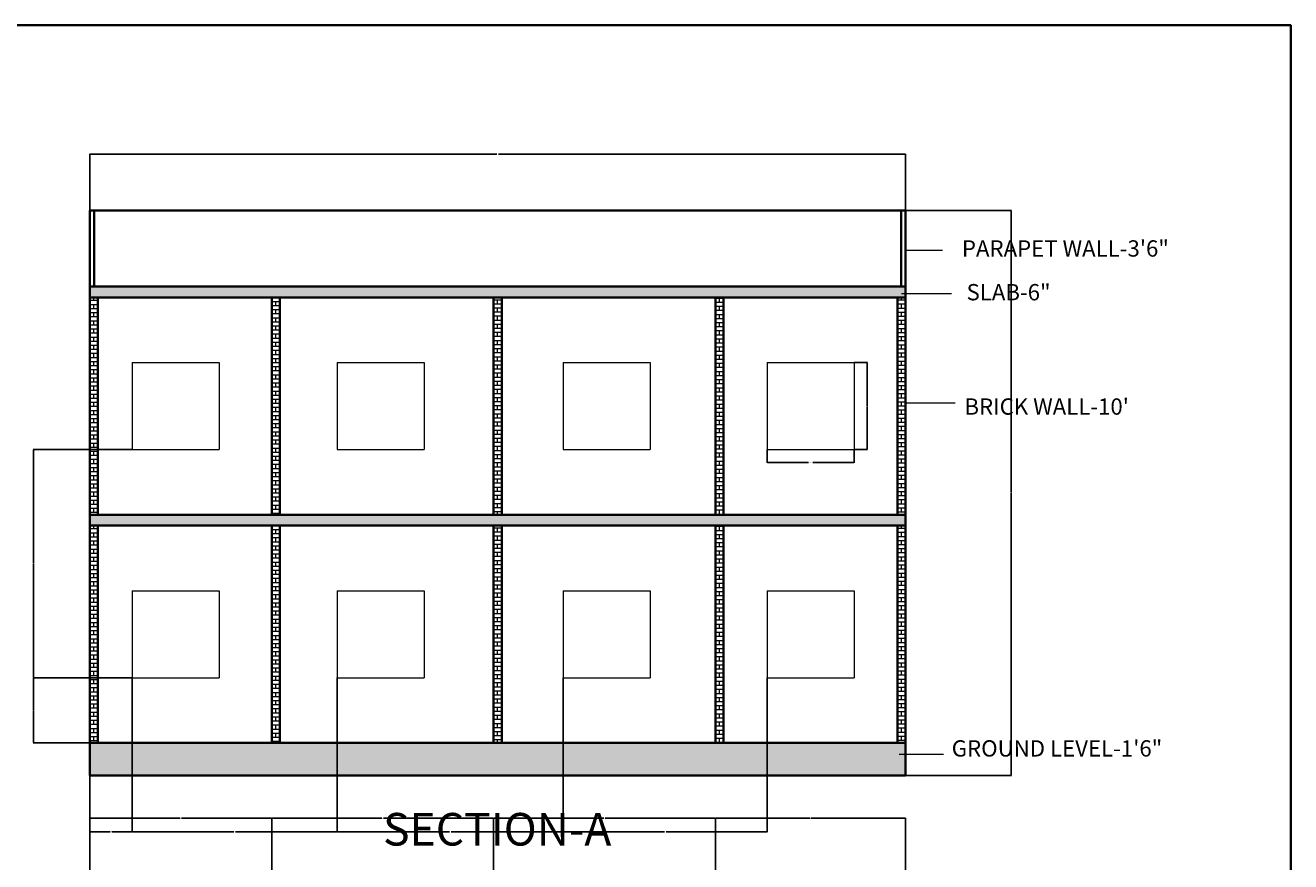
# Model space of a CAD drawing. Units: inches. Extents: x 2043 to 3387, y 1535 to 2797.
# Tile 7 of 7: x 2688 to 3387, y 2335 to 2797. Entities that reach past the tile are written whole.
import ezdxf

# ---------------------------------------------------------------- set-up
doc = ezdxf.new("R2010")
doc.units = ezdxf.units.IN
for name, color, linetype, lineweight in [('A-ANNO-DIMS', 2, 'Continuous', 18), ('A-ANNO-TEXT', 7, 'Continuous', 18), ('A-ANNO-TITL', 7, 'Continuous', 30), ('A-ANNO-TTLB', 7, 'Continuous', 35), ('A-GLAZ', 4, 'Continuous', 18), ('A-SECT', 7, 'Continuous', 35), ('A-WALL-PATT', 8, 'Continuous', 13), ('S-CONC-PATT', 8, 'Continuous', 13)]:
    doc.layers.add(name, color=color, linetype=linetype, lineweight=lineweight)
doc.styles.get("Standard").update_dxf_attribs({"font": 'arial.ttf'})
doc.dimstyles.get("Standard").update_dxf_attribs({"dimtxt": 0.18, "dimasz": 0.18, "dimexe": 0.18, "dimexo": 0.0625, "dimgap": 0.09, "dimtad": 0, "dimtih": 1, "dimtoh": 1, "dimdec": 4, "dimzin": 0, "dimdsep": 46, "dimtxsty": 'Standard', "dimcen": 0.09, "dimadec": 0, "dimazin": 0, "dimtfac": 1, "dimtdec": 4, "dimtofl": 0, "dimtmove": 0, "dimatfit": 3, "dimfxl": 1, "dimtolj": 1, "dimtzin": 0, "dimarcsym": 0})

# ---------------------------------------------------------------- blocks, each defined once
blk = doc.blocks.new('WIN-48-SECTION')
for p, q in [((0, 48), (48, 48)), ((0, 48), (0, 0)), ((48, 48), (48, 0)), ((0, 0), (48, 0))]:
    blk.add_line(p, q)
blk = doc.blocks.new('*D47')
at = {"layer": 'A-ANNO-DIMS', "color": 0, "lineweight": -2, "transparency": 16777216}
for p, q in [((3097.86, 2562.49), (3097.86, 2555.17)), ((3145.86, 2562.49), (3145.86, 2555.17)), ((3098.04, 2555.35), (3120.72, 2555.35)), ((3145.68, 2555.35), (3123, 2555.35))]:
    blk.add_line(p, q, dxfattribs=at)
at = {"layer": 'A-ANNO-DIMS', "color": 0, "transparency": 16777216}
for points in [[(3098.04, 2555.38), (3098.04, 2555.32), (3097.86, 2555.35)], [(3145.68, 2555.38), (3145.68, 2555.32), (3145.86, 2555.35)]]:
    blk.add_solid(points, dxfattribs=at)
at = {"layer": 'Defpoints', "color": 0, "transparency": 16777216}
for p in [(3097.86, 2562.55), (3145.86, 2562.55), (3145.86, 2555.35)]:
    blk.add_point(p, dxfattribs=at)
at = {"layer": 'A-ANNO-DIMS', "color": 0, "transparency": 16777216, "insert": (3121.86, 2555.35), "char_height": 0.18, "attachment_point": 5}
blk.add_mtext('\\A1;OPENING 48 TYP.', dxfattribs=at)
blk = doc.blocks.new('*D48')
at = {"layer": 'A-ANNO-DIMS', "color": 0, "lineweight": -2, "transparency": 16777216}
for p, q in [((3145.92, 2610.55), (3153.24, 2610.55)), ((3153.06, 2610.37), (3153.06, 2586.73)), ((3153.06, 2562.73), (3153.06, 2586.37)), ((3145.92, 2562.55), (3153.24, 2562.55))]:
    blk.add_line(p, q, dxfattribs=at)
at = {"layer": 'A-ANNO-DIMS', "color": 0, "transparency": 16777216}
for points in [[(3153.03, 2610.37), (3153.09, 2610.37), (3153.06, 2610.55)], [(3153.03, 2562.73), (3153.09, 2562.73), (3153.06, 2562.55)]]:
    blk.add_solid(points, dxfattribs=at)
at = {"layer": 'Defpoints', "color": 0, "transparency": 16777216}
for p in [(3145.86, 2610.55), (3153.06, 2610.55), (3145.86, 2562.55)]:
    blk.add_point(p, dxfattribs=at)
at = {"layer": 'A-ANNO-DIMS', "color": 0, "transparency": 16777216, "insert": (3153.06, 2586.55), "char_height": 0.18, "attachment_point": 5}
blk.add_mtext('\\A1;48 TYP.', dxfattribs=at)
blk = doc.blocks.new('*D107')
at = {"layer": 'A-ANNO-DIMS', "color": 0, "lineweight": -2, "transparency": 16777216}
for p, q in [((2723.71, 2326.44), (2723.71, 2359.26)), ((2723.89, 2359.08), (2773.57, 2359.08)), ((2824.03, 2359.08), (2774.34, 2359.08)), ((2824.21, 2317.44), (2824.21, 2359.26))]:
    blk.add_line(p, q, dxfattribs=at)
at = {"layer": 'A-ANNO-DIMS', "color": 0, "transparency": 16777216}
for points in [[(2723.89, 2359.11), (2723.89, 2359.05), (2723.71, 2359.08)], [(2824.03, 2359.11), (2824.03, 2359.05), (2824.21, 2359.08)]]:
    blk.add_solid(points, dxfattribs=at)
at = {"layer": 'Defpoints', "color": 0, "transparency": 16777216}
for p in [(2824.21, 2359.08), (2723.71, 2326.38), (2824.21, 2317.38)]:
    blk.add_point(p, dxfattribs=at)
at = {"layer": 'A-ANNO-DIMS', "color": 0, "transparency": 16777216, "insert": (2773.96, 2359.08), "char_height": 0.18, "attachment_point": 5}
blk.add_mtext('\\A1;100.5', dxfattribs=at)
blk = doc.blocks.new('*D108')
at = {"layer": 'A-ANNO-DIMS', "color": 0, "lineweight": -2, "transparency": 16777216}
for p, q in [((2824.21, 2317.44), (2824.21, 2359.26)), ((2824.39, 2359.08), (2885.07, 2359.08)), ((2946.53, 2359.08), (2885.84, 2359.08)), ((2946.71, 2317.44), (2946.71, 2359.26))]:
    blk.add_line(p, q, dxfattribs=at)
at = {"layer": 'A-ANNO-DIMS', "color": 0, "transparency": 16777216}
for points in [[(2824.39, 2359.11), (2824.39, 2359.05), (2824.21, 2359.08)], [(2946.53, 2359.11), (2946.53, 2359.05), (2946.71, 2359.08)]]:
    blk.add_solid(points, dxfattribs=at)
at = {"layer": 'Defpoints', "color": 0, "transparency": 16777216}
for p in [(2946.71, 2359.08), (2824.21, 2317.38), (2946.71, 2317.38)]:
    blk.add_point(p, dxfattribs=at)
at = {"layer": 'A-ANNO-DIMS', "color": 0, "transparency": 16777216, "insert": (2885.46, 2359.08), "char_height": 0.18, "attachment_point": 5}
blk.add_mtext('\\A1;122.5', dxfattribs=at)
blk = doc.blocks.new('*D109')
at = {"layer": 'A-ANNO-DIMS', "color": 0, "lineweight": -2, "transparency": 16777216}
for p, q in [((2946.71, 2317.44), (2946.71, 2359.26)), ((2946.89, 2359.08), (3007.57, 2359.08)), ((3069.03, 2359.08), (3008.34, 2359.08)), ((3069.21, 2317.44), (3069.21, 2359.26))]:
    blk.add_line(p, q, dxfattribs=at)
at = {"layer": 'A-ANNO-DIMS', "color": 0, "transparency": 16777216}
for points in [[(2946.89, 2359.11), (2946.89, 2359.05), (2946.71, 2359.08)], [(3069.03, 2359.11), (3069.03, 2359.05), (3069.21, 2359.08)]]:
    blk.add_solid(points, dxfattribs=at)
at = {"layer": 'Defpoints', "color": 0, "transparency": 16777216}
for p in [(3069.21, 2359.08), (2946.71, 2317.38), (3069.21, 2317.38)]:
    blk.add_point(p, dxfattribs=at)
at = {"layer": 'A-ANNO-DIMS', "color": 0, "transparency": 16777216, "insert": (3007.96, 2359.08), "char_height": 0.18, "attachment_point": 5}
blk.add_mtext('\\A1;122.5', dxfattribs=at)
blk = doc.blocks.new('*D110')
at = {"layer": 'A-ANNO-DIMS', "color": 0, "lineweight": -2, "transparency": 16777216}
for p, q in [((3069.21, 2317.44), (3069.21, 2359.26)), ((3069.39, 2359.08), (3121.43, 2359.08)), ((3174.03, 2359.08), (3121.99, 2359.08)), ((3174.21, 2326.44), (3174.21, 2359.26))]:
    blk.add_line(p, q, dxfattribs=at)
at = {"layer": 'A-ANNO-DIMS', "color": 0, "transparency": 16777216}
for points in [[(3069.39, 2359.11), (3069.39, 2359.05), (3069.21, 2359.08)], [(3174.03, 2359.11), (3174.03, 2359.05), (3174.21, 2359.08)]]:
    blk.add_solid(points, dxfattribs=at)
at = {"layer": 'Defpoints', "color": 0, "transparency": 16777216}
for p in [(3174.21, 2359.08), (3174.21, 2326.38), (3069.21, 2317.38)]:
    blk.add_point(p, dxfattribs=at)
at = {"layer": 'A-ANNO-DIMS', "color": 0, "transparency": 16777216, "insert": (3121.71, 2359.08), "char_height": 0.18, "attachment_point": 5}
blk.add_mtext('\\A1;105', dxfattribs=at)
blk = doc.blocks.new('*D120')
at = {"layer": 'A-ANNO-DIMS', "color": 0, "lineweight": -2, "transparency": 16777216}
for p, q in [((2723.71, 2694.61), (2723.71, 2725.78)), ((3174.21, 2694.61), (3174.21, 2725.78)), ((2723.89, 2725.6), (2948.56, 2725.6)), ((3174.03, 2725.6), (2949.36, 2725.6))]:
    blk.add_line(p, q, dxfattribs=at)
at = {"layer": 'A-ANNO-DIMS', "color": 0, "transparency": 16777216}
for points in [[(2723.89, 2725.63), (2723.89, 2725.57), (2723.71, 2725.6)], [(3174.03, 2725.63), (3174.03, 2725.57), (3174.21, 2725.6)]]:
    blk.add_solid(points, dxfattribs=at)
at = {"layer": 'Defpoints', "color": 0, "transparency": 16777216}
for p in [(3174.21, 2725.6), (2723.71, 2694.55), (3174.21, 2694.55)]:
    blk.add_point(p, dxfattribs=at)
at = {"layer": 'A-ANNO-DIMS', "color": 0, "transparency": 16777216, "insert": (2948.96, 2725.6), "char_height": 0.18, "attachment_point": 5}
blk.add_mtext('\\A1;450.5', dxfattribs=at)
blk = doc.blocks.new('*D121')
at = {"layer": 'A-ANNO-DIMS', "color": 0, "lineweight": -2, "transparency": 16777216}
for p, q in [((3174.27, 2694.55), (3232.83, 2694.55)), ((3232.65, 2694.37), (3232.65, 2538.73)), ((3232.65, 2382.73), (3232.65, 2538.37)), ((3174.27, 2382.55), (3232.83, 2382.55))]:
    blk.add_line(p, q, dxfattribs=at)
at = {"layer": 'A-ANNO-DIMS', "color": 0, "transparency": 16777216}
for points in [[(3232.62, 2694.37), (3232.68, 2694.37), (3232.65, 2694.55)], [(3232.62, 2382.73), (3232.68, 2382.73), (3232.65, 2382.55)]]:
    blk.add_solid(points, dxfattribs=at)
at = {"layer": 'Defpoints', "color": 0, "transparency": 16777216}
for p in [(3174.21, 2694.55), (3232.65, 2694.55), (3174.21, 2382.55)]:
    blk.add_point(p, dxfattribs=at)
at = {"layer": 'A-ANNO-DIMS', "color": 0, "transparency": 16777216, "insert": (3232.65, 2538.55), "char_height": 0.18, "attachment_point": 5}
blk.add_mtext('\\A1;312', dxfattribs=at)
blk = doc.blocks.new('*D127')
at = {"layer": 'A-ANNO-DIMS', "color": 0, "lineweight": -2, "transparency": 16777216}
for p, q in [((2747.01, 2562.55), (2692.48, 2562.55)), ((2692.66, 2562.37), (2692.66, 2499.73)), ((2692.66, 2436.73), (2692.66, 2499.37)), ((2747.01, 2436.55), (2692.48, 2436.55))]:
    blk.add_line(p, q, dxfattribs=at)
at = {"layer": 'A-ANNO-DIMS', "color": 0, "transparency": 16777216}
for points in [[(2692.63, 2562.37), (2692.69, 2562.37), (2692.66, 2562.55)], [(2692.63, 2436.73), (2692.69, 2436.73), (2692.66, 2436.55)]]:
    blk.add_solid(points, dxfattribs=at)
at = {"layer": 'Defpoints', "color": 0, "transparency": 16777216}
for p in [(2692.66, 2562.55), (2747.07, 2562.55), (2747.07, 2436.55)]:
    blk.add_point(p, dxfattribs=at)
at = {"layer": 'A-ANNO-DIMS', "color": 0, "transparency": 16777216, "insert": (2692.66, 2499.55), "char_height": 0.18, "attachment_point": 5}
blk.add_mtext('\\A1;126', dxfattribs=at)
blk = doc.blocks.new('*D128')
at = {"layer": 'A-ANNO-DIMS', "color": 0, "lineweight": -2, "transparency": 16777216}
for p, q in [((2747.07, 2436.49), (2747.07, 2351.32)), ((2723.71, 2400.49), (2723.71, 2351.32)), ((2723.89, 2351.5), (2734.99, 2351.5)), ((2746.89, 2351.5), (2735.78, 2351.5))]:
    blk.add_line(p, q, dxfattribs=at)
at = {"layer": 'A-ANNO-DIMS', "color": 0, "transparency": 16777216}
for points in [[(2723.89, 2351.53), (2723.89, 2351.47), (2723.71, 2351.5)], [(2746.89, 2351.53), (2746.89, 2351.47), (2747.07, 2351.5)]]:
    blk.add_solid(points, dxfattribs=at)
at = {"layer": 'Defpoints', "color": 0, "transparency": 16777216}
for p in [(2747.07, 2436.55), (2723.71, 2400.55), (2747.07, 2351.5)]:
    blk.add_point(p, dxfattribs=at)
at = {"layer": 'A-ANNO-DIMS', "color": 0, "transparency": 16777216, "insert": (2735.39, 2351.5), "char_height": 0.18, "attachment_point": 5}
blk.add_mtext('\\A1;23.36', dxfattribs=at)
blk = doc.blocks.new('*D129')
at = {"layer": 'A-ANNO-DIMS', "color": 0, "lineweight": -2, "transparency": 16777216}
for p, q in [((2747.07, 2436.49), (2747.07, 2351.32)), ((2860.38, 2436.49), (2860.38, 2351.32)), ((2747.25, 2351.5), (2803.29, 2351.5)), ((2860.2, 2351.5), (2804.16, 2351.5))]:
    blk.add_line(p, q, dxfattribs=at)
at = {"layer": 'A-ANNO-DIMS', "color": 0, "transparency": 16777216}
for points in [[(2747.25, 2351.53), (2747.25, 2351.47), (2747.07, 2351.5)], [(2860.2, 2351.53), (2860.2, 2351.47), (2860.38, 2351.5)]]:
    blk.add_solid(points, dxfattribs=at)
at = {"layer": 'Defpoints', "color": 0, "transparency": 16777216}
for p in [(2747.07, 2436.55), (2860.38, 2436.55), (2860.38, 2351.5)]:
    blk.add_point(p, dxfattribs=at)
at = {"layer": 'A-ANNO-DIMS', "color": 0, "transparency": 16777216, "insert": (2803.73, 2351.5), "char_height": 0.18, "attachment_point": 5}
blk.add_mtext('\\A1;113.31', dxfattribs=at)
blk = doc.blocks.new('*D130')
at = {"layer": 'A-ANNO-DIMS', "color": 0, "lineweight": -2, "transparency": 16777216}
for p, q in [((2860.38, 2436.49), (2860.38, 2351.32)), ((2985.21, 2436.49), (2985.21, 2351.32)), ((2860.56, 2351.5), (2922.34, 2351.5)), ((2985.03, 2351.5), (2923.25, 2351.5))]:
    blk.add_line(p, q, dxfattribs=at)
at = {"layer": 'A-ANNO-DIMS', "color": 0, "transparency": 16777216}
for points in [[(2860.56, 2351.53), (2860.56, 2351.47), (2860.38, 2351.5)], [(2985.03, 2351.53), (2985.03, 2351.47), (2985.21, 2351.5)]]:
    blk.add_solid(points, dxfattribs=at)
at = {"layer": 'Defpoints', "color": 0, "transparency": 16777216}
for p in [(2860.38, 2436.55), (2985.21, 2436.55), (2985.21, 2351.5)]:
    blk.add_point(p, dxfattribs=at)
at = {"layer": 'A-ANNO-DIMS', "color": 0, "transparency": 16777216, "insert": (2922.8, 2351.5), "char_height": 0.18, "attachment_point": 5}
blk.add_mtext('\\A1;124.83', dxfattribs=at)
blk = doc.blocks.new('*D131')
at = {"layer": 'A-ANNO-DIMS', "color": 0, "lineweight": -2, "transparency": 16777216}
for p, q in [((2985.21, 2436.49), (2985.21, 2351.32)), ((3097.86, 2436.49), (3097.86, 2351.32)), ((2985.39, 2351.5), (3041.08, 2351.5)), ((3097.68, 2351.5), (3041.99, 2351.5))]:
    blk.add_line(p, q, dxfattribs=at)
at = {"layer": 'A-ANNO-DIMS', "color": 0, "transparency": 16777216}
for points in [[(2985.39, 2351.53), (2985.39, 2351.47), (2985.21, 2351.5)], [(3097.68, 2351.53), (3097.68, 2351.47), (3097.86, 2351.5)]]:
    blk.add_solid(points, dxfattribs=at)
at = {"layer": 'Defpoints', "color": 0, "transparency": 16777216}
for p in [(2985.21, 2436.55), (3097.86, 2436.55), (3097.86, 2351.5)]:
    blk.add_point(p, dxfattribs=at)
at = {"layer": 'A-ANNO-DIMS', "color": 0, "transparency": 16777216, "insert": (3041.54, 2351.5), "char_height": 0.18, "attachment_point": 5}
blk.add_mtext('\\A1;112.65', dxfattribs=at)
blk = doc.blocks.new('*D132')
at = {"layer": 'A-ANNO-DIMS', "color": 0, "lineweight": -2, "transparency": 16777216}
for p, q in [((2747.01, 2436.55), (2692.48, 2436.55)), ((2692.66, 2436.37), (2692.66, 2418.73)), ((2692.66, 2400.73), (2692.66, 2418.37)), ((2723.65, 2400.55), (2692.48, 2400.55))]:
    blk.add_line(p, q, dxfattribs=at)
at = {"layer": 'A-ANNO-DIMS', "color": 0, "transparency": 16777216}
for points in [[(2692.63, 2436.37), (2692.69, 2436.37), (2692.66, 2436.55)], [(2692.63, 2400.73), (2692.69, 2400.73), (2692.66, 2400.55)]]:
    blk.add_solid(points, dxfattribs=at)
at = {"layer": 'Defpoints', "color": 0, "transparency": 16777216}
for p in [(2747.07, 2436.55), (2692.66, 2400.55), (2723.71, 2400.55)]:
    blk.add_point(p, dxfattribs=at)
at = {"layer": 'A-ANNO-DIMS', "color": 0, "transparency": 16777216, "insert": (2692.66, 2418.55), "char_height": 0.18, "attachment_point": 5}
blk.add_mtext('\\A1;36', dxfattribs=at)

msp = doc.modelspace()

# ---------------------------------------------------------------- hatches: boundary and pattern name
at = {"layer": 'A-WALL-PATT'}
h = msp.add_hatch(dxfattribs=at)
h.set_pattern_fill('BRICK', color=256, scale=0.354488, style=0)
h.paths.add_polyline_path([(2723.7086, 2526.549), (2728.2086, 2526.549), (2728.2086, 2646.549), (2723.7086, 2646.549)])
h = msp.add_hatch(dxfattribs=at)
h.set_pattern_fill('BRICK', color=256, scale=0.354106, style=0)
h.paths.add_polyline_path([(2824.2086, 2526.549), (2828.7086, 2526.549), (2828.7086, 2646.549), (2824.2086, 2646.549)])
h = msp.add_hatch(dxfattribs=at)
h.set_pattern_fill('BRICK', color=256, scale=0.3542356, style=0)
h.paths.add_polyline_path([(2946.7086, 2526.549), (2951.2086, 2526.549), (2951.2086, 2646.549), (2946.7086, 2646.549)])
h = msp.add_hatch(dxfattribs=at)
h.set_pattern_fill('BRICK', color=256, scale=0.3543548, style=0)
h.paths.add_polyline_path([(3069.2086, 2526.549), (3073.7086, 2526.549), (3073.7086, 2646.549), (3069.2086, 2646.549)])
h = msp.add_hatch(dxfattribs=at)
h.set_pattern_fill('BRICK', color=256, scale=0.354522, style=0)
h.paths.add_polyline_path([(3169.7086, 2526.549), (3174.2086, 2526.549), (3174.2086, 2646.549), (3169.7086, 2646.549)])
h = msp.add_hatch(dxfattribs=at)
h.set_pattern_fill('BRICK', color=256, scale=0.354488, style=0)
h.paths.add_polyline_path([(2723.7086, 2400.549), (2728.2086, 2400.549), (2728.2086, 2520.549), (2723.7086, 2520.549)])
h = msp.add_hatch(dxfattribs=at)
h.set_pattern_fill('BRICK', color=256, scale=0.354106, style=0)
h.paths.add_polyline_path([(2824.2086, 2400.549), (2828.7086, 2400.549), (2828.7086, 2520.549), (2824.2086, 2520.549)])
h = msp.add_hatch(dxfattribs=at)
h.set_pattern_fill('BRICK', color=256, scale=0.3542356, style=0)
h.paths.add_polyline_path([(2946.7086, 2400.549), (2951.2086, 2400.549), (2951.2086, 2520.549), (2946.7086, 2520.549)])
h = msp.add_hatch(dxfattribs=at)
h.set_pattern_fill('BRICK', color=256, scale=0.3543548, style=0)
h.paths.add_polyline_path([(3069.2086, 2400.549), (3073.7086, 2400.549), (3073.7086, 2520.549), (3069.2086, 2520.549)])
h = msp.add_hatch(dxfattribs=at)
h.set_pattern_fill('BRICK', color=256, scale=0.354522, style=0)
h.paths.add_polyline_path([(3169.7086, 2400.549), (3174.2086, 2400.549), (3174.2086, 2520.549), (3169.7086, 2520.549)])
at = {"layer": 'S-CONC-PATT'}
h = msp.add_hatch(dxfattribs=at)
h.set_pattern_fill('AR-CONC', color=256, scale=0.046, style=0)
h.paths.add_polyline_path([(2723.7086, 2646.549), (3174.2086, 2646.549), (3174.2086, 2652.549), (2723.7086, 2652.549)])
h = msp.add_hatch(dxfattribs=at)
h.set_pattern_fill('AR-CONC', color=256, scale=0.046, style=0)
h.paths.add_polyline_path([(2723.7086, 2520.549), (3174.2086, 2520.549), (3174.2086, 2526.549), (2723.7086, 2526.549)])
h = msp.add_hatch(dxfattribs=at)
h.set_pattern_fill('AR-CONC', color=256, scale=0.081, style=0)
h.paths.add_polyline_path([(2723.7086, 2382.549), (3174.2086, 2382.549), (3174.2086, 2400.549), (2723.7086, 2400.549)])

# ---------------------------------------------------------------- linework, layer by layer
at = {"layer": 'A-ANNO-TEXT'}
for p, q in [((3174.2086, 2672.5466), (3194.7465, 2672.5466)), ((3171.9586, 2648.7305), (3199.698, 2648.7305)), ((3174.2086, 2588.2999), (3201.6035, 2588.2999)), ((3170.6746, 2394.3592), (3195.2013, 2394.3592))]:
    msp.add_line(p, q, dxfattribs=at)
at = {"layer": 'A-ANNO-TTLB'}
msp.add_lwpolyline([(2042.5541, 2796.7818), (3386.9704, 2796.7818), (3386.9704, 1534.5689), (2042.5541, 1534.5689)], close=True, dxfattribs=at)
at = {"layer": 'A-SECT'}
for p, q in [((2723.7086, 2694.549), (2723.7086, 2508.549)), ((2723.7086, 2694.549), (3174.2086, 2694.549)), ((2726.1278, 2652.549), (2726.1278, 2694.549)), ((3171.8877, 2652.549), (3171.8877, 2694.549)), ((3174.2086, 2694.549), (3174.2086, 2508.549)), ((2723.7086, 2652.549), (3174.2086, 2652.549)), ((2723.7086, 2646.549), (3174.2086, 2646.549)), ((2728.2086, 2646.549), (2728.2086, 2526.549)), ((2728.2086, 2646.549), (2728.2086, 2526.549)), ((2824.2086, 2646.549), (2824.2086, 2526.549)), ((2828.7086, 2646.549), (2828.7086, 2526.549)), ((2946.7086, 2646.549), (2946.7086, 2526.549)), ((2951.2086, 2646.549), (2951.2086, 2526.549)), ((3069.2086, 2646.549), (3069.2086, 2526.549)), ((3073.7086, 2646.549), (3073.7086, 2526.549)), ((3169.7086, 2526.549), (3169.7086, 2646.549)), ((2723.7086, 2568.549), (2723.7086, 2382.549)), ((3174.2086, 2568.549), (3174.2086, 2382.549)), ((2723.7086, 2526.549), (3174.2086, 2526.549)), ((2723.7086, 2520.549), (3174.2086, 2520.549)), ((2728.2086, 2520.549), (2728.2086, 2400.549)), ((2728.2086, 2520.549), (2728.2086, 2400.549)), ((2824.2086, 2520.549), (2824.2086, 2400.549)), ((2828.7086, 2520.549), (2828.7086, 2400.549)), ((2946.7086, 2520.549), (2946.7086, 2400.549)), ((2951.2086, 2520.549), (2951.2086, 2400.549)), ((3069.2086, 2520.549), (3069.2086, 2400.549)), ((3073.7086, 2520.549), (3073.7086, 2400.549)), ((3169.7086, 2400.549), (3169.7086, 2520.549)), ((2723.7086, 2400.549), (3174.2086, 2400.549)), ((2723.7086, 2382.549), (3174.2086, 2382.549))]:
    msp.add_line(p, q, dxfattribs=at)

# ---------------------------------------------------------------- block references
at = {"layer": 'A-GLAZ'}
for p in [(2747.069, 2562.549), (2860.3827, 2562.549), (2985.2127, 2562.549), (3097.8621, 2562.549), (2747.069, 2436.549), (2860.3827, 2436.549), (2985.2127, 2436.549), (3097.8621, 2436.549)]:
    msp.add_blockref('WIN-48-SECTION', p, dxfattribs=at)

# ---------------------------------------------------------------- texts
at = {"layer": 'A-ANNO-TEXT', "char_height": 9, "attachment_point": 1}
for s, width, insert in [('PARAPET WALL-3\'6"', 372.310488, (3205.3781, 2678.063)), ('SLAB-6"', 39.654642, (3207.9357, 2653.9192)), ("BRICK WALL-10'", 111.749552, (3206.7623, 2590.7785)), ('GROUND LEVEL-1\'6"', 169.236647, (3199.7479, 2402.0126))]:
    msp.add_mtext_dynamic_manual_height_columns(s, width=width, gutter_width=12.5, heights=[0], dxfattribs=dict(at, insert=insert))
at = {"layer": 'A-ANNO-TITL', "insert": (2885.6627, 2361.8667), "char_height": 18, "attachment_point": 1}
msp.add_mtext_dynamic_manual_height_columns('SECTION-A', width=189.460503, gutter_width=12.5, heights=[0], dxfattribs=at)

# ---------------------------------------------------------------- dimensions: what is measured, and where the dimension line sits
at = {"layer": 'A-ANNO-DIMS'}
for base, p1, p2, override, picture, middle in [((3174.2086, 2725.599), (2723.7086, 2694.549), (3174.2086, 2694.549), {"dimdec": 1, "dimlfac": 1, "dimrnd": 0, "dimzin": 0, "dimdsep": 46, "dimlunit": 2}, '*D120', (2948.9586, 2725.599)), ((2747.0692, 2351.499), (2723.7086, 2400.549), (2747.0692, 2436.549), {"dimdec": 2, "dimlfac": 1, "dimrnd": 0, "dimzin": 0, "dimdsep": 46, "dimlunit": 2}, '*D128', (2735.3889, 2351.499)), ((2860.3829, 2351.499), (2747.0692, 2436.549), (2860.3829, 2436.549), {"dimdec": 2, "dimlfac": 1, "dimrnd": 0, "dimzin": 0, "dimdsep": 46, "dimlunit": 2}, '*D129', (2803.726, 2351.499)), ((2985.2128, 2351.499), (2860.3829, 2436.549), (2985.2128, 2436.549), {"dimdec": 2, "dimlfac": 1, "dimrnd": 0, "dimzin": 0, "dimdsep": 46, "dimlunit": 2}, '*D130', (2922.7979, 2351.499)), ((3097.8623, 2351.499), (2985.2128, 2436.549), (3097.8623, 2436.549), {"dimdec": 2, "dimlfac": 1, "dimrnd": 0, "dimzin": 0, "dimdsep": 46, "dimlunit": 2}, '*D131', (3041.5376, 2351.499)), ((2824.2086, 2359.0769), (2723.7086, 2326.3769), (2824.2086, 2317.3769), {"dimdec": 1, "dimlfac": 1, "dimrnd": 0, "dimzin": 0, "dimdsep": 46, "dimlunit": 2}, '*D107', (2773.9586, 2359.0769)), ((2946.7086, 2359.0769), (2824.2086, 2317.3769), (2946.7086, 2317.3769), {"dimdec": 1, "dimlfac": 1, "dimrnd": 0, "dimzin": 0, "dimdsep": 46, "dimlunit": 2}, '*D108', (2885.4586, 2359.0769)), ((3069.2086, 2359.0769), (2946.7086, 2317.3769), (3069.2086, 2317.3769), {"dimdec": 1, "dimlfac": 1, "dimrnd": 0, "dimzin": 0, "dimdsep": 46, "dimlunit": 2}, '*D109', (3007.9586, 2359.0769)), ((3174.2086, 2359.0769), (3069.2086, 2317.3769), (3174.2086, 2326.3769), {"dimdec": 0, "dimlfac": 1, "dimrnd": 0, "dimzin": 0, "dimdsep": 46, "dimlunit": 2}, '*D110', (3121.7086, 2359.0769))]:
    dim = msp.add_linear_dim(base=base, p1=p1, p2=p2, dimstyle='Standard', override=override, dxfattribs=at)
    dim.commit()
    dim.dimension.update_dxf_attribs({"geometry": picture, "text_midpoint": middle})
for base, p1, p2, picture, middle in [((3232.6535, 2694.549), (3174.2086, 2382.549), (3174.2086, 2694.549), '*D121', (3232.6535, 2538.549)), ((2692.6586, 2562.549), (2747.0692, 2436.549), (2747.0692, 2562.549), '*D127', (2692.6586, 2499.549)), ((2692.6586, 2400.549), (2747.0692, 2436.549), (2723.7086, 2400.549), '*D132', (2692.6586, 2418.549))]:
    dim = msp.add_linear_dim(base=base, p1=p1, p2=p2, angle=90, dimstyle='Standard', override={"dimdec": 0, "dimlfac": 1, "dimrnd": 0, "dimzin": 0, "dimdsep": 46, "dimlunit": 2}, dxfattribs=at)
    dim.commit()
    dim.dimension.update_dxf_attribs({"geometry": picture, "text_midpoint": middle})
dim = msp.add_linear_dim(base=(3153.0623, 2610.549), p1=(3145.8623, 2562.549), p2=(3145.8623, 2610.549), angle=90, text='<> TYP.', dimstyle='Standard', override={"dimdec": 0, "dimlfac": 1, "dimrnd": 0, "dimzin": 0, "dimdsep": 46, "dimlunit": 2}, dxfattribs=at)
dim.commit()
dim.dimension.update_dxf_attribs({"geometry": '*D48', "text_midpoint": (3153.0623, 2586.549)})
dim = msp.add_linear_dim(base=(3145.8623, 2555.349), p1=(3097.8623, 2562.549), p2=(3145.8623, 2562.549), text='OPENING <> TYP.', dimstyle='Standard', override={"dimdec": 0, "dimlfac": 1, "dimrnd": 0, "dimzin": 0, "dimdsep": 46, "dimlunit": 2}, dxfattribs=at)
dim.commit()
dim.dimension.update_dxf_attribs({"geometry": '*D47', "text_midpoint": (3121.8623, 2555.349)})

doc.saveas('drawing.dxf')
